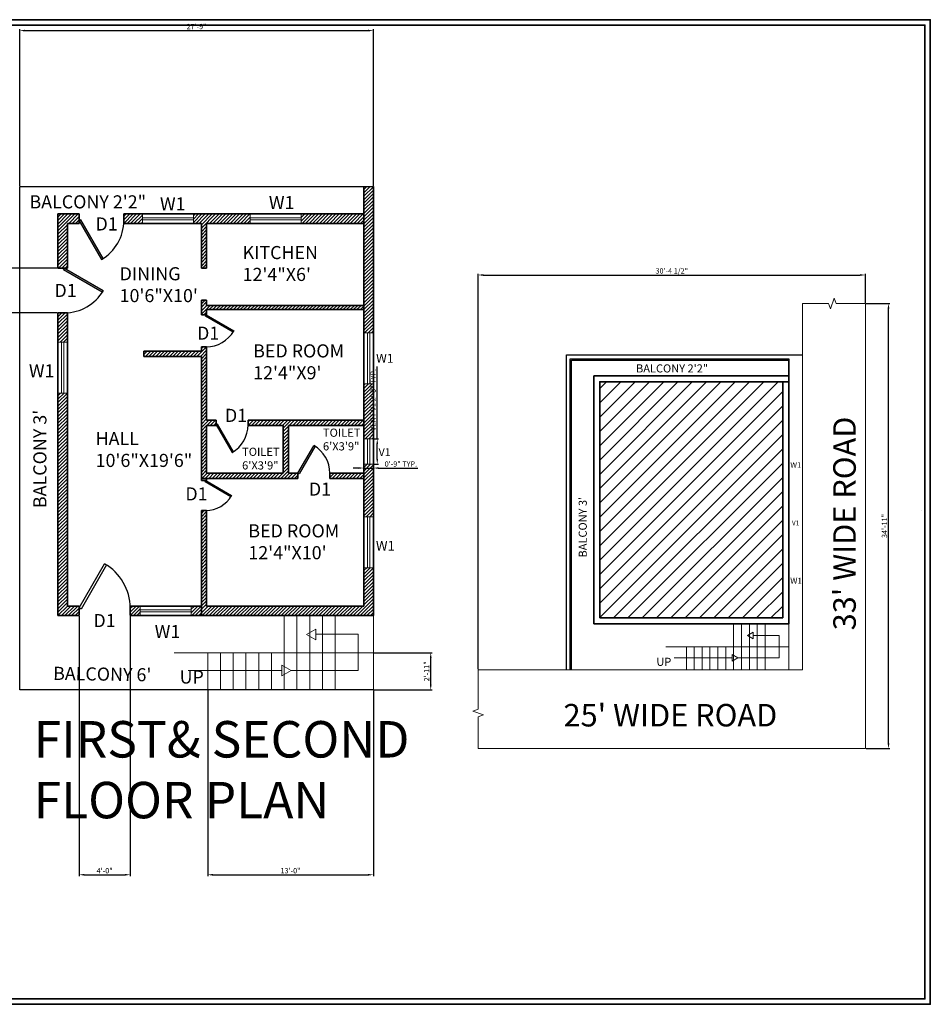
# Model space of a CAD drawing. Units: inches. Extents: x 2257 to 3849, y 1105 to 2032.
# Tile 2 of 2: x 2992 to 3849, y 1105 to 2032. Entities that reach past the tile are written whole.
import ezdxf

# ---------------------------------------------------------------- set-up
doc = ezdxf.new("R2010")
doc.units = ezdxf.units.IN
for name, color, linetype, lineweight in [('A-ANNO-DIMS', 7, 'Continuous', 18), ('A-ANNO-SYMB', 7, 'Continuous', 18), ('A-ANNO-TEXT', 130, 'Continuous', 18), ('A-ANNO-TTLB', 7, 'Continuous', 35), ('A-AREA-IDEN', 130, 'Continuous', 18), ('A-FLOR-OTLN', 7, 'Continuous', 25), ('C-PROP', 7, 'Continuous', 25), ('C-ROAD', 7, 'Continuous', 18), ('Doors', 100, 'Continuous', 25), ('steps', 220, 'Continuous', 18), ('walls', 10, 'Continuous', 35), ('windows', 160, 'Continuous', 18)]:
    doc.layers.add(name, color=color, linetype=linetype, lineweight=lineweight)
doc.layers.add('A-ROOF-PATT', color=51, linetype='Continuous', lineweight=13, true_color=0xf8f6b0)
doc.layers.add('A-WALL-PATT', color=241, linetype='Continuous', lineweight=13, true_color=0xf7abae)
doc.styles.get("Standard").update_dxf_attribs({"font": 'arial.ttf'})
doc.dimstyles.new('ISO-25', dxfattribs={"dimtxt": 5, "dimasz": 5, "dimexe": 1.25, "dimexo": 0.625, "dimtad": 1, "dimlunit": 3, "dimtxsty": 'Standard', "dimcen": 2.5, "dimadec": 0, "dimazin": 0, "dimtfac": 1, "dimtmove": 0, "dimatfit": 3, "dimfxl": 1, "dimarcsym": 0})
pattern_1 = [(45, (-85.9454, 0), (-1.6164461, 1.6164461), [])]

# ---------------------------------------------------------------- blocks, each defined once
blk = doc.blocks.new('*U4')
for p, q in [((0, 0), (0, -6)), ((40, 0), (40, -6))]:
    blk.add_line(p, q)
blk.add_lwpolyline([(0, 0), (20, 34.64), (21.52, 33.77), (1.52, -0.88)], close=True)
blk.add_arc((0, 0), 40, 0, 60)
blk = doc.blocks.new('*U5')
for p, q in [((-40, 0), (-40, 6)), ((0, 0), (0, 6))]:
    blk.add_line(p, q)
blk.add_lwpolyline([(0, 0), (-20, -34.64), (-21.52, -33.77), (-1.52, 0.87)], close=True)
blk.add_arc((0, 0), 40, 180, 240)
blk = doc.blocks.new('*U6')
for p, q in [((0, 0), (0, -6)), ((-40, 0), (-40, -6))]:
    blk.add_line(p, q)
blk.add_lwpolyline([(0, 0), (-20, 34.64), (-21.52, 33.77), (-1.52, -0.88)], close=True)
blk.add_arc((0, 0), 40, 120, 180)
blk = doc.blocks.new('*U7')
for p, q in [((-40, 0), (-40, 6)), ((0, 0), (0, 6))]:
    blk.add_line(p, q)
blk.add_lwpolyline([(0, 0), (-20, -34.6), (-21.5, -33.8), (-1.5, 0.9)], close=True)
blk.add_arc((0, 0), 40, 180, 240)
blk = doc.blocks.new('WIN-W1-48IN')
for p, q in [((0, 5.5), (48, 5.5)), ((0, 3.5), (48, 3.5))]:
    blk.add_line(p, q)
blk.add_lwpolyline([(0, 9), (48, 9), (48, 0), (0, 0)], close=True)
blk = doc.blocks.new('VENT-V1-24IN')
for p, q in [((3.5, 0), (3.5, 24)), ((5.5, 0), (5.5, 24))]:
    blk.add_line(p, q)
blk.add_lwpolyline([(0, 0), (0, 24), (9, 24), (9, 0)], close=True)
blk = doc.blocks.new('STAIR-DIRECTION-RETURN')
for points in [[(96.97, 5.1), (160.01, 5.1), (160.01, 39.11), (120.14, 39.11)], [(0, 5.1), (88.35, 5.1)]]:
    blk.add_lwpolyline(points)
for points in [[(120.14, 34.02), (120.14, 44.09), (111.42, 39.05)], [(88.35, 10.07), (88.35, 0), (97.07, 5.03)]]:
    blk.add_lwpolyline(points, close=True)
blk = doc.blocks.new('*D20')
at = {"layer": 'A-ANNO-DIMS', "color": 0, "lineweight": -2, "transparency": 16777216}
for p, q in [((3328.33, 1637.83), (3328.33, 1705.87)), ((3325.36, 1637.83), (3329.58, 1637.83)), ((3328.33, 1618.83), (3328.33, 1632.83)), ((3325.36, 1613.83), (3329.58, 1613.83))]:
    blk.add_line(p, q, dxfattribs=at)
at = {"layer": 'A-ANNO-DIMS', "color": 0, "transparency": 16777216}
for points in [[(3327.5, 1632.83), (3329.16, 1632.83), (3328.33, 1637.83)], [(3327.5, 1618.83), (3329.16, 1618.83), (3328.33, 1613.83)]]:
    blk.add_solid(points, dxfattribs=at)
at = {"layer": 'DEFPOINTS', "color": 0, "transparency": 16777216}
for p in [(3324.73, 1637.83), (3328.33, 1637.83), (3324.73, 1613.83)]:
    blk.add_point(p, dxfattribs=at)
at = {"layer": 'A-ANNO-DIMS', "color": 0, "transparency": 16777216, "insert": (3325.15, 1674.35), "char_height": 5, "attachment_point": 5, "rotation": 90}
blk.add_mtext('VENT V1 2\'-0" TYP.', dxfattribs=at)
blk = doc.blocks.new('*D21')
at = {"layer": 'A-ANNO-DIMS', "color": 0, "lineweight": -2, "transparency": 16777216}
for p, q in [((3315.73, 1613.2), (3315.73, 1608.98)), ((3324.73, 1613.2), (3324.73, 1608.98)), ((3310.73, 1610.23), (3305.73, 1610.23)), ((3315.73, 1610.23), (3324.73, 1610.23)), ((3329.73, 1610.23), (3366.46, 1610.23))]:
    blk.add_line(p, q, dxfattribs=at)
at = {"layer": 'A-ANNO-DIMS', "color": 0, "transparency": 16777216}
for points in [[(3310.73, 1611.06), (3310.73, 1609.39), (3315.73, 1610.23)], [(3329.73, 1611.06), (3329.73, 1609.39), (3324.73, 1610.23)]]:
    blk.add_solid(points, dxfattribs=at)
at = {"layer": 'DEFPOINTS', "color": 0, "transparency": 16777216}
for p in [(3315.73, 1613.83), (3324.73, 1613.83), (3324.73, 1610.23)]:
    blk.add_point(p, dxfattribs=at)
at = {"layer": 'A-ANNO-DIMS', "color": 0, "transparency": 16777216, "insert": (3350.6, 1613.4), "char_height": 5, "attachment_point": 5}
blk.add_mtext('0\'-9" TYP.', dxfattribs=at)
blk = doc.blocks.new('*D22')
at = {"layer": 'A-ANNO-DIMS', "color": 0, "lineweight": -2, "transparency": 16777216}
for p, q in [((2991.73, 1875.97), (2991.73, 2023.22)), ((2996.73, 2021.97), (3319.73, 2021.97)), ((3324.73, 1875.97), (3324.73, 2023.22))]:
    blk.add_line(p, q, dxfattribs=at)
at = {"layer": 'A-ANNO-DIMS', "color": 0, "transparency": 16777216}
for points in [[(2996.73, 2022.81), (2996.73, 2021.14), (2991.73, 2021.97)], [(3319.73, 2022.81), (3319.73, 2021.14), (3324.73, 2021.97)]]:
    blk.add_solid(points, dxfattribs=at)
at = {"layer": 'DEFPOINTS', "color": 0, "transparency": 16777216}
for p in [(3324.73, 2021.97), (2991.73, 1875.35), (3324.73, 1875.35)]:
    blk.add_point(p, dxfattribs=at)
at = {"layer": 'A-ANNO-DIMS', "color": 0, "transparency": 16777216, "insert": (3158.23, 2025.15), "char_height": 5, "attachment_point": 5}
blk.add_mtext('27\'-9"', dxfattribs=at)
blk = doc.blocks.new('*D24')
at = {"layer": 'A-ANNO-DIMS', "color": 0, "lineweight": -2, "transparency": 16777216}
for p, q in [((3047.73, 1470.72), (3047.73, 1226.15)), ((3095.73, 1470.72), (3095.73, 1226.15)), ((3052.73, 1227.4), (3090.73, 1227.4))]:
    blk.add_line(p, q, dxfattribs=at)
at = {"layer": 'A-ANNO-DIMS', "color": 0, "transparency": 16777216}
for points in [[(3052.73, 1228.23), (3052.73, 1226.56), (3047.73, 1227.4)], [(3090.73, 1228.23), (3090.73, 1226.56), (3095.73, 1227.4)]]:
    blk.add_solid(points, dxfattribs=at)
at = {"layer": 'DEFPOINTS', "color": 0, "transparency": 16777216}
for p in [(3047.73, 1471.35), (3095.73, 1471.35), (3095.73, 1227.4)]:
    blk.add_point(p, dxfattribs=at)
at = {"layer": 'A-ANNO-DIMS', "color": 0, "transparency": 16777216, "insert": (3071.73, 1230.57), "char_height": 5, "attachment_point": 5}
blk.add_mtext('4\'-0"', dxfattribs=at)
blk = doc.blocks.new('*D25')
at = {"layer": 'A-ANNO-DIMS', "color": 0, "lineweight": -2, "transparency": 16777216}
for p, q in [((3027.11, 1798.35), (2262.98, 1798.35)), ((2264.23, 1761.35), (2264.23, 1793.35)), ((3027.11, 1756.35), (2262.98, 1756.35))]:
    blk.add_line(p, q, dxfattribs=at)
at = {"layer": 'A-ANNO-DIMS', "color": 0, "transparency": 16777216}
for points in [[(2263.39, 1793.35), (2265.06, 1793.35), (2264.23, 1798.35)], [(2263.39, 1761.35), (2265.06, 1761.35), (2264.23, 1756.35)]]:
    blk.add_solid(points, dxfattribs=at)
at = {"layer": 'DEFPOINTS', "color": 0, "transparency": 16777216}
for p in [(2264.23, 1798.35), (3027.73, 1798.35), (3027.73, 1756.35)]:
    blk.add_point(p, dxfattribs=at)
at = {"layer": 'A-ANNO-DIMS', "color": 0, "transparency": 16777216, "insert": (2261.05, 1777.35), "char_height": 5, "attachment_point": 5, "rotation": 90}
blk.add_mtext('3\'-6"', dxfattribs=at)
blk = doc.blocks.new('*D28')
at = {"layer": 'A-ANNO-DIMS', "color": 0, "lineweight": -2, "transparency": 16777216}
for p, q in [((3168.73, 1400.72), (3168.73, 1226.15)), ((3324.73, 1400.72), (3324.73, 1226.15)), ((3173.73, 1227.4), (3319.73, 1227.4))]:
    blk.add_line(p, q, dxfattribs=at)
at = {"layer": 'A-ANNO-DIMS', "color": 0, "transparency": 16777216}
for points in [[(3173.73, 1228.23), (3173.73, 1226.56), (3168.73, 1227.4)], [(3319.73, 1228.23), (3319.73, 1226.56), (3324.73, 1227.4)]]:
    blk.add_solid(points, dxfattribs=at)
at = {"layer": 'DEFPOINTS', "color": 0, "transparency": 16777216}
for p in [(3168.73, 1401.35), (3324.73, 1401.35), (3324.73, 1227.4)]:
    blk.add_point(p, dxfattribs=at)
at = {"layer": 'A-ANNO-DIMS', "color": 0, "transparency": 16777216, "insert": (3246.73, 1230.58), "char_height": 5, "attachment_point": 5}
blk.add_mtext('13\'-0"', dxfattribs=at)
blk = doc.blocks.new('*D29')
at = {"layer": 'A-ANNO-DIMS', "color": 0, "lineweight": -2, "transparency": 16777216}
for p, q in [((3325.36, 1436.35), (3379.93, 1436.35)), ((3378.68, 1406.35), (3378.68, 1431.35)), ((3325.36, 1401.35), (3379.93, 1401.35))]:
    blk.add_line(p, q, dxfattribs=at)
at = {"layer": 'A-ANNO-DIMS', "color": 0, "transparency": 16777216}
for points in [[(3377.85, 1431.35), (3379.51, 1431.35), (3378.68, 1436.35)], [(3377.85, 1406.35), (3379.51, 1406.35), (3378.68, 1401.35)]]:
    blk.add_solid(points, dxfattribs=at)
at = {"layer": 'DEFPOINTS', "color": 0, "transparency": 16777216}
for p in [(3324.73, 1436.35), (3378.68, 1436.35), (3324.73, 1401.35)]:
    blk.add_point(p, dxfattribs=at)
at = {"layer": 'A-ANNO-DIMS', "color": 0, "transparency": 16777216, "insert": (3375.55, 1418.85), "char_height": 5, "attachment_point": 5, "rotation": 90}
blk.add_mtext('2\'-11"', dxfattribs=at)
blk = doc.blocks.new('*D30')
at = {"layer": 'A-ANNO-DIMS', "color": 0, "lineweight": -2, "transparency": 16777216}
for p, q in [((3423.28, 1420.92), (3423.28, 1793.17)), ((3428.28, 1791.92), (3782.92, 1791.92)), ((3787.92, 1765.76), (3787.92, 1793.17))]:
    blk.add_line(p, q, dxfattribs=at)
at = {"layer": 'A-ANNO-DIMS', "color": 0, "transparency": 16777216}
for points in [[(3428.28, 1792.76), (3428.28, 1791.09), (3423.28, 1791.92)], [(3782.92, 1792.76), (3782.92, 1791.09), (3787.92, 1791.92)]]:
    blk.add_solid(points, dxfattribs=at)
at = {"layer": 'DEFPOINTS', "color": 0, "transparency": 16777216}
for p in [(3787.92, 1791.92), (3787.92, 1765.13), (3423.28, 1420.3)]:
    blk.add_point(p, dxfattribs=at)
at = {"layer": 'A-ANNO-DIMS', "color": 0, "transparency": 16777216, "insert": (3605.6, 1795.14), "char_height": 5, "attachment_point": 5}
blk.add_mtext('30\'-4 1/2"', dxfattribs=at)
blk = doc.blocks.new('*D31')
at = {"layer": 'A-ANNO-DIMS', "color": 0, "lineweight": -2, "transparency": 16777216}
for p, q in [((3788.55, 1765.13), (3810.87, 1765.13)), ((3809.62, 1351.2), (3809.62, 1760.13)), ((3788.55, 1346.2), (3810.87, 1346.2))]:
    blk.add_line(p, q, dxfattribs=at)
at = {"layer": 'A-ANNO-DIMS', "color": 0, "transparency": 16777216}
for points in [[(3808.79, 1760.13), (3810.46, 1760.13), (3809.62, 1765.13)], [(3808.79, 1351.2), (3810.46, 1351.2), (3809.62, 1346.2)]]:
    blk.add_solid(points, dxfattribs=at)
at = {"layer": 'DEFPOINTS', "color": 0, "transparency": 16777216}
for p in [(3787.92, 1765.13), (3809.62, 1765.13), (3787.92, 1346.2)]:
    blk.add_point(p, dxfattribs=at)
at = {"layer": 'A-ANNO-DIMS', "color": 0, "transparency": 16777216, "insert": (3806.44, 1555.67), "char_height": 5, "attachment_point": 5, "rotation": 90}
blk.add_mtext('34\'-11"', dxfattribs=at)

msp = doc.modelspace()

# ---------------------------------------------------------------- hatches: boundary and pattern name
at = {"layer": 'A-ROOF-PATT'}
h = msp.add_hatch(dxfattribs=at)
h.set_pattern_fill('ANSI31', color=256, scale=3)
h.set_pattern_definition([(45, (-221.724, 0), (-6.735192, 6.735192), [])])
h.paths.add_polyline_path([(3710.119, 1469.082), (3710.119, 1691.383), (3537.836, 1691.383), (3537.836, 1665.448), (3537.836, 1469.082)])
at = {"layer": 'A-WALL-PATT'}
h = msp.add_hatch(dxfattribs=at)
h.set_pattern_fill('ANSI31', color=256, scale=0.72)
h.set_pattern_definition(pattern_1)
h.paths.add_polyline_path([(3036.731, 1840.347), (3047.731, 1840.347), (3047.731, 1849.347), (3027.731, 1849.347), (3027.731, 1798.347), (3036.731, 1798.347)])
h.paths.add_polyline_path([(3107.208, 1849.347), (3089.731, 1849.347), (3089.731, 1840.347), (3107.208, 1840.347)])
h.paths.add_polyline_path([(3208.789, 1849.347), (3155.208, 1849.347), (3155.208, 1840.347), (3162.731, 1840.347), (3162.731, 1798.347), (3167.731, 1798.347), (3167.731, 1840.347), (3208.789, 1840.347)])
h.paths.add_polyline_path([(3315.731, 1849.347), (3256.789, 1849.347), (3256.789, 1840.347), (3315.731, 1840.347)])
h.paths.add_polyline_path([(3324.731, 1875.347), (3315.731, 1875.347), (3315.731, 1737.469), (3324.731, 1737.469)])
h.paths.add_polyline_path([(3167.731, 1768.347), (3162.731, 1768.347), (3162.731, 1754.347), (3167.231, 1754.347), (3167.731, 1754.347), (3167.731, 1759.347), (3315.731, 1759.347), (3315.731, 1763.347), (3167.731, 1763.347)])
h.paths.add_polyline_path([(3167.731, 1724.347), (3162.731, 1724.347), (3162.731, 1720.347), (3108.731, 1720.347), (3108.731, 1715.347), (3162.731, 1715.347), (3162.731, 1600.347), (3167.731, 1600.347), (3253.731, 1600.347), (3253.731, 1605.347), (3244.731, 1605.347), (3244.731, 1650.347), (3315.731, 1650.347), (3315.731, 1655.347), (3206.731, 1655.347), (3206.731, 1650.347), (3239.731, 1650.347), (3239.731, 1605.347), (3167.731, 1605.347), (3167.731, 1650.347), (3176.731, 1650.347), (3176.731, 1655.347), (3167.731, 1655.347)])
h.paths.add_polyline_path([(3324.731, 1689.469), (3315.731, 1689.469), (3315.731, 1637.826), (3324.731, 1637.826)])
h.paths.add_polyline_path([(3315.731, 1605.347), (3283.731, 1605.347), (3283.731, 1600.347), (3315.731, 1600.347)], flags=17)
h.paths.add_polyline_path([(3324.731, 1613.826), (3315.731, 1613.826), (3315.731, 1564.439), (3324.731, 1564.439)])
h.paths.add_polyline_path([(3324.731, 1516.439), (3315.731, 1516.439), (3315.731, 1480.347), (3167.731, 1480.347), (3167.731, 1570.347), (3162.731, 1570.347), (3162.731, 1471.347), (3324.731, 1471.347)])
h.paths.add_polyline_path([(3162.731, 1480.347), (3153.231, 1480.347), (3153.231, 1471.347), (3162.731, 1471.347)])
h.paths.add_polyline_path([(3105.231, 1480.347), (3095.731, 1480.347), (3095.731, 1471.347), (3105.231, 1471.347)])
h = msp.add_hatch(dxfattribs=at)
h.set_pattern_fill('ANSI31', color=256, scale=0.72)
h.set_pattern_definition(pattern_1)
h.paths.add_polyline_path([(2551.998, 1559.347), (2542.498, 1559.347), (2542.498, 1550.347), (2551.998, 1550.347)])
h.paths.add_polyline_path([(2494.498, 1559.347), (2484.998, 1559.347), (2484.998, 1550.347), (2494.498, 1550.347)])
h.paths.add_polyline_path([(3036.731, 1680.812), (3027.731, 1680.812), (3027.731, 1471.347), (3047.694, 1471.347), (3047.694, 1478.53), (3047.731, 1480.347), (3036.731, 1480.347)])
h.paths.add_polyline_path([(3036.731, 1756.347), (3027.731, 1756.347), (3027.731, 1728.812), (3036.731, 1728.812)])
h = msp.add_hatch(dxfattribs=at)
h.set_pattern_fill('ANSI31', color=256, scale=0.72)
h.set_pattern_definition(pattern_1)
h.paths.add_polyline_path([(3036.731, 1756.347), (3027.731, 1756.347), (3027.731, 1728.812), (3036.731, 1728.812)])

# ---------------------------------------------------------------- linework, layer by layer
at = {"layer": 'A-ANNO-SYMB'}
for points in [[(3728.644, 1765.134), (3753.039, 1765.134), (3754.892, 1760.044), (3758.597, 1770.223), (3760.449, 1765.134), (3787.924, 1765.134)], [(3667.811, 1431.653), (3706.737, 1431.653), (3706.737, 1452.659), (3682.121, 1452.659)], [(3607.932, 1431.653), (3662.491, 1431.653)], [(3423.275, 1420.3), (3423.275, 1383.369), (3418.186, 1381.517), (3428.365, 1377.812), (3423.275, 1375.959), (3423.275, 1346.199)]]:
    msp.add_lwpolyline(points, dxfattribs=at)
for points in [[(3682.121, 1449.512), (3682.121, 1455.731), (3676.735, 1452.621)], [(3662.491, 1434.724), (3662.491, 1428.506), (3667.876, 1431.615)]]:
    msp.add_lwpolyline(points, close=True, dxfattribs=at)
at = {"layer": 'A-ANNO-TTLB'}
for points in [[(2257.449, 2032.239), (3848.988, 2032.239), (3848.988, 1105.467), (2257.449, 1105.467)], [(2262.449, 2027.239), (3843.988, 2027.239), (3843.988, 1110.467), (2262.449, 1110.467)]]:
    msp.add_lwpolyline(points, close=True, dxfattribs=at)
at = {"layer": 'A-FLOR-OTLN'}
for p, q in [((2991.731, 1875.347), (3324.731, 1875.347)), ((2991.731, 1401.347), (2991.731, 1875.347)), ((3510.048, 1420.3), (3510.048, 1712.996)), ((3510.048, 1712.996), (3715.677, 1712.996)), ((3324.731, 1401.347), (2991.731, 1401.347))]:
    msp.add_line(p, q, dxfattribs=at)
msp.add_lwpolyline([(3511.283, 1420.3), (3511.283, 1711.761), (3715.677, 1711.761)], dxfattribs=at)
at = {"layer": 'C-PROP'}
for p, q in [((3506.343, 1420.3), (3506.343, 1716.701)), ((3506.343, 1716.701), (3728.644, 1716.701))]:
    msp.add_line(p, q, dxfattribs=at)
at = {"layer": 'C-ROAD'}
for p, q in [((3728.644, 1765.134), (3728.644, 1420.3)), ((3787.924, 1765.134), (3787.924, 1346.199)), ((3728.644, 1420.3), (3423.275, 1420.3)), ((3787.924, 1346.199), (3423.275, 1346.199))]:
    msp.add_line(p, q, dxfattribs=at)
at = {"layer": 'steps'}
for p, q in [((3240.731, 1471.347), (3240.731, 1401.347)), ((3252.731, 1471.347), (3252.731, 1401.347)), ((3252.731, 1471.347), (3252.731, 1401.347)), ((3264.731, 1471.347), (3264.731, 1401.347)), ((3276.731, 1471.347), (3276.731, 1401.347)), ((3288.731, 1471.347), (3288.731, 1401.347)), ((3324.731, 1471.347), (3324.731, 1401.347)), ((3663.806, 1463.525), (3663.806, 1420.3)), ((3678.626, 1463.525), (3678.626, 1420.3)), ((3686.037, 1463.525), (3686.037, 1420.3)), ((3693.447, 1463.525), (3693.447, 1420.3)), ((3715.677, 1463.525), (3715.677, 1420.3)), ((3599.931, 1441.912), (3715.677, 1441.912)), ((3619.346, 1441.912), (3619.346, 1420.3)), ((3626.756, 1441.912), (3626.756, 1420.3)), ((3634.166, 1441.912), (3634.166, 1420.3)), ((3641.576, 1441.912), (3641.576, 1420.3)), ((3648.986, 1441.912), (3648.986, 1420.3)), ((3656.396, 1441.912), (3656.396, 1420.3)), ((3137.29, 1436.347), (3324.731, 1436.347)), ((3168.731, 1436.347), (3168.731, 1401.347)), ((3180.731, 1436.347), (3180.731, 1401.347)), ((3192.731, 1436.347), (3192.731, 1401.347)), ((3204.731, 1436.347), (3204.731, 1401.347)), ((3216.731, 1436.347), (3216.731, 1401.347)), ((3228.731, 1436.347), (3228.731, 1401.347))]:
    msp.add_line(p, q, dxfattribs=at)
msp.add_lwpolyline([(3671.216, 1463.525), (3671.216, 1420.3)], close=True, dxfattribs=at)
at = {"layer": 'walls'}
for p, q in [((3315.731, 1875.347), (3315.731, 1480.347)), ((3324.731, 1875.347), (3324.731, 1471.347)), ((3027.731, 1849.347), (3047.731, 1849.347)), ((3027.731, 1798.347), (3027.731, 1849.347)), ((3047.731, 1840.347), (3047.731, 1849.347)), ((3089.731, 1849.347), (3315.731, 1849.347)), ((3089.731, 1840.347), (3089.731, 1849.347)), ((3036.731, 1840.347), (3047.731, 1840.347)), ((3036.731, 1798.347), (3036.731, 1840.347)), ((3089.731, 1840.347), (3162.731, 1840.347)), ((3162.731, 1798.347), (3162.731, 1840.347)), ((3167.731, 1840.347), (3167.731, 1798.347)), ((3167.731, 1840.347), (3315.731, 1840.347)), ((3027.731, 1798.347), (3036.731, 1798.347)), ((3162.731, 1798.347), (3167.731, 1798.347)), ((3162.731, 1768.347), (3167.731, 1768.347)), ((3162.731, 1754.347), (3162.731, 1768.347)), ((3167.731, 1768.347), (3167.731, 1763.347)), ((3167.731, 1763.347), (3315.731, 1763.347)), ((3027.731, 1756.347), (3036.731, 1756.347)), ((3027.731, 1471.347), (3027.731, 1756.347)), ((3036.731, 1480.347), (3036.731, 1756.347)), ((3162.731, 1754.347), (3167.731, 1754.347)), ((3167.731, 1759.347), (3315.731, 1759.347)), ((3167.731, 1759.347), (3167.731, 1754.347)), ((3162.731, 1724.347), (3167.731, 1724.347)), ((3162.731, 1720.347), (3162.731, 1724.347)), ((3167.731, 1724.347), (3167.731, 1655.347)), ((3108.731, 1720.347), (3162.731, 1720.347)), ((3108.731, 1715.347), (3108.731, 1720.347)), ((3108.731, 1715.347), (3162.731, 1715.347)), ((3162.731, 1600.347), (3162.731, 1715.347)), ((3715.677, 1712.996), (3715.677, 1463.525)), ((3710.119, 1691.383), (3710.119, 1469.082)), ((3167.731, 1655.347), (3176.731, 1655.347)), ((3167.731, 1650.347), (3176.731, 1650.347)), ((3167.731, 1650.347), (3167.731, 1605.347)), ((3176.731, 1655.347), (3176.731, 1650.347)), ((3206.731, 1655.347), (3315.731, 1655.347)), ((3206.731, 1655.347), (3206.731, 1650.347)), ((3206.731, 1650.347), (3239.731, 1650.347)), ((3239.731, 1650.347), (3239.731, 1605.347)), ((3244.731, 1650.347), (3244.731, 1605.347)), ((3244.731, 1650.347), (3315.731, 1650.347)), ((3167.731, 1605.347), (3239.731, 1605.347)), ((3244.731, 1605.347), (3253.731, 1605.347)), ((3253.731, 1605.347), (3253.731, 1600.347)), ((3283.731, 1605.347), (3315.731, 1605.347)), ((3283.731, 1605.347), (3283.731, 1600.347)), ((3162.731, 1600.347), (3253.731, 1600.347)), ((3162.731, 1600.347), (3167.731, 1600.347)), ((3162.731, 1600.347), (3162.731, 1598.347)), ((3162.731, 1598.347), (3167.731, 1598.347)), ((3167.731, 1598.347), (3167.731, 1600.347)), ((3283.731, 1600.347), (3315.731, 1600.347)), ((3162.731, 1570.347), (3167.731, 1570.347)), ((3162.731, 1471.347), (3162.731, 1570.347)), ((3167.731, 1570.347), (3167.731, 1480.347)), ((3036.731, 1480.347), (3047.731, 1480.347)), ((3047.731, 1471.347), (3047.731, 1480.347)), ((3095.731, 1480.347), (3162.731, 1480.347)), ((3095.731, 1471.347), (3095.731, 1480.347)), ((3167.731, 1480.347), (3315.731, 1480.347)), ((3027.731, 1471.347), (3047.731, 1471.347)), ((3095.731, 1471.347), (3162.731, 1471.347)), ((3162.731, 1471.347), (3324.731, 1471.347)), ((3710.119, 1469.082), (3537.836, 1469.082)), ((3715.677, 1463.525), (3532.278, 1463.525))]:
    msp.add_line(p, q, dxfattribs=at)
for points in [[(3532.278, 1696.941), (3532.278, 1463.525)], [(3544.628, 1696.941), (3532.278, 1696.941), (3532.278, 1665.448)], [(3532.278, 1592.87), (3532.278, 1696.941)], [(3537.836, 1696.941), (3715.677, 1696.941)], [(3715.677, 1691.383), (3537.836, 1691.383)], [(3537.836, 1665.448), (3537.836, 1691.383), (3544.628, 1691.383)], [(3537.836, 1469.082), (3537.836, 1691.383)], [(3537.836, 1622.511), (3537.836, 1639.513)]]:
    msp.add_lwpolyline(points, dxfattribs=at)
at = {"layer": 'windows'}
for p, q in [((3031.231, 1680.812), (3031.231, 1728.812)), ((3033.231, 1680.812), (3033.231, 1728.812))]:
    msp.add_line(p, q, dxfattribs=at)
for points in [[(3027.731, 1680.812), (3027.731, 1728.812), (3036.731, 1728.812), (3036.731, 1680.812)], [(3840.593, 1570.605), (3840.593, 1570.605)]]:
    msp.add_lwpolyline(points, close=True, dxfattribs=at)

# ---------------------------------------------------------------- block references
at = {"layer": 'A-ANNO-SYMB'}
msp.add_blockref('STAIR-DIRECTION-RETURN', (3150.247, 1414.636), dxfattribs=at)
at = {"layer": 'Doors'}
for name, p, xscale, yscale, zscale, rotation in [('*U6', (3047.731, 1843.047), 1.049999999999999, 1.049999999999999, 1.049999999999999, 180), ('*U5', (3034.031, 1798.347), 1.049999999999999, 1.049999999999999, 1.049999999999999, 90), ('*U5', (3167.231, 1754.347), 0.75, 0.75, 0.75, 90), ('*U6', (3176.731, 1650.849), 0.7496246408594235, 0.7496246408594235, 0.7496246408594235, 180), ('*U7', (3253.731, 1605.347), 0.7496246408594235, 0.7496246408594235, 0.7496246408594235, 180), ('*U5', (3166.931, 1598.347), 0.6999999999999944, 0.6999999999999944, 0.6999999999999944, 90)]:
    msp.add_blockref(name, p, dxfattribs=dict(at, xscale=xscale, yscale=yscale, zscale=zscale, rotation=rotation))
at = {"layer": 'Doors', "xscale": 1.200942847219647, "yscale": 1.200942847219647, "zscale": 1.200942847219647}
msp.add_blockref('*U4', (3047.694, 1478.53), dxfattribs=at)
at = {"layer": 'windows'}
for name, p in [('WIN-W1-48IN', (3107.207, 1840.347)), ('WIN-W1-48IN', (3208.789, 1840.347)), ('VENT-V1-24IN', (3315.731, 1613.826)), ('WIN-W1-48IN', (3105.231, 1471.347))]:
    msp.add_blockref(name, p, dxfattribs=at)
for p, rotation in [((3324.731, 1689.469), 89.99999999999923), ((3324.731, 1516.439), 89.99999999999905)]:
    msp.add_blockref('WIN-W1-48IN', p, dxfattribs=dict(at, rotation=rotation))

# ---------------------------------------------------------------- texts
at = {"layer": 'A-ANNO-TEXT', "attachment_point": 1}
for s, width, gutter_width, insert, char_height in [('W1', 167.82029, 61.663, (3123.769, 1865.042), 12.3325), ('W1', 167.82029, 61.663, (3226.304, 1866.238), 12.3325), ('D1', 167.82029, 61.663, (3063.102, 1846.134), 12.3325), ('D1', 167.82029, 61.663, (3024.457, 1783.521), 12.3325), ('D1', 167.82029, 61.663, (3158.715, 1743.35), 12.3325), ('W1', 114.48409, 42.065, (3327.262, 1717.711), 8.413), ('W1', 167.82029, 61.663, (3000.401, 1707.912), 12.3325), ('D1', 167.82029, 61.663, (3184.947, 1665.964), 12.3325), ('V1', 100.10563, 36.782, (3329.599, 1628.888), 7.3564), ('W1', 70.69423, 25.975, (3717.24, 1615.655), 5.1951), ('D1', 167.82029, 61.663, (3263.962, 1596.568), 12.3325), ('D1', 167.82029, 61.663, (3147.704, 1592.042), 12.3325), ('V1', 61.8155, 22.713, (3718.682, 1560.807), 4.5426), ('W1', 124.29149, 45.669, (3327.091, 1541.615), 9.1337), ('W1', 76.75033, 28.201, (3717.134, 1506.916), 5.6401), ('D1', 167.82029, 61.663, (3061.139, 1472.812), 12.3325), ('W1', 167.82029, 61.663, (3118.81, 1462.459), 12.3325), ('UP', 103.62948, 38.077, (3591.126, 1431.653), 7.6154), ('UP', 167.82029, 61.663, (3142.281, 1419.732), 12.3325), ("25' WIDE ROAD", 288.40348, 105.969, (3503.733, 1388.191), 21.19372), ('FIRST& SECOND FLOOR PLAN', 467.04814, 171.608, (3004.915, 1372.061), 34.32167)]:
    msp.add_mtext_dynamic_manual_height_columns(s, width=width, gutter_width=gutter_width, heights=[0], dxfattribs=dict(at, insert=insert, char_height=char_height))
at = {"layer": 'A-ANNO-TEXT', "insert": (3757.627, 1457.47), "char_height": 21.19372, "attachment_point": 1, "rotation": 90}
msp.add_mtext_dynamic_manual_height_columns("33' WIDE ROAD", width=288.40348, gutter_width=105.969, heights=[0], dxfattribs=at)
at = {"layer": 'A-AREA-IDEN', "attachment_point": 1}
for s, width, gutter_width, insert, char_height in [('BALCONY 2\'2"', 254.30567, 61.663, (3000.93, 1866.935), 12.3325), ('KITCHEN \\P12\'4"X6\'', 167.82029, 61.663, (3201.588, 1819.217), 12.3325), ('DINING \\P10\'6"X10\'', 167.82029, 61.663, (3085.81, 1799.256), 12.3325), ('BED ROOM\\P12\'4"X9\'', 167.82029, 61.663, (3211.518, 1726.65), 12.3325), ('BALCONY 2\'2"', 157.03443, 38.077, (3571.956, 1707.802), 7.61535), ('HALL \\P10\'6"X19\'6"', 167.82029, 61.663, (3063.217, 1644.142), 12.3325), ('TOILET\\P6\'X3\'9"', 104.71521, 38.476, (3277.225, 1647.35), 7.6951), ('TOILET\\P6\'X3\'9"', 104.71521, 38.476, (3201.091, 1629.38), 7.6951), ('BED ROOM  \\P12\'4"X10\'', 167.82029, 61.663, (3206.987, 1557.279), 12.3325)]:
    msp.add_mtext_dynamic_manual_height_columns(s, width=width, gutter_width=gutter_width, heights=[0], dxfattribs=dict(at, insert=insert, char_height=char_height))
for s, width, gutter_width, insert, char_height, rotation in [("BALCONY 3'", 254.30567, 61.663, (3004.586, 1572.53), 12.3325, 90), ("BALCONY 3'", 157.03443, 38.077, (3517.986, 1526.006), 7.6154, 90), ("BALCONY 6'", 254.30567, 61.663, (3023.295, 1423.212), 12.3325, 359.068345)]:
    msp.add_mtext_dynamic_manual_height_columns(s, width=width, gutter_width=gutter_width, heights=[0], dxfattribs=dict(at, insert=insert, char_height=char_height, rotation=rotation))

# ---------------------------------------------------------------- dimensions: what is measured, and where the dimension line sits
at = {"layer": 'A-ANNO-DIMS'}
for base, p1, p2, picture, middle in [((3324.731, 2021.972), (2991.731, 1875.347), (3324.731, 1875.347), '*D22', (3158.231, 2025.15)), ((3787.924, 1791.923), (3423.275, 1420.3), (3787.924, 1765.134), '*D30', (3605.6, 1795.135)), ((3095.731, 1227.397), (3047.731, 1471.347), (3095.731, 1471.347), '*D24', (3071.731, 1230.574)), ((3324.731, 1227.397), (3168.731, 1401.347), (3324.731, 1401.347), '*D28', (3246.731, 1230.576))]:
    dim = msp.add_linear_dim(base=base, p1=p1, p2=p2, dimstyle='ISO-25', override={"dimdec": 1, "dimlfac": 1, "dimrnd": 0, "dimzin": 1, "dimdsep": 46, "dimlunit": 4, "dimfrac": 2}, dxfattribs=at)
    dim.commit()
    dim.dimension.update_dxf_attribs({"geometry": picture, "text_midpoint": middle})
for base, p1, p2, picture, middle in [((2264.228, 1798.347), (3027.731, 1756.347), (3027.731, 1798.347), '*D25', (2261.049, 1777.347)), ((3809.624, 1765.134), (3787.924, 1346.199), (3787.924, 1765.134), '*D31', (3806.445, 1555.666)), ((3378.681, 1436.347), (3324.731, 1401.347), (3324.731, 1436.347), '*D29', (3375.546, 1418.847))]:
    dim = msp.add_linear_dim(base=base, p1=p1, p2=p2, angle=90, dimstyle='ISO-25', override={"dimdec": 1, "dimlfac": 1, "dimrnd": 0, "dimzin": 1, "dimdsep": 46, "dimlunit": 4, "dimfrac": 2}, dxfattribs=at)
    dim.commit()
    dim.dimension.update_dxf_attribs({"geometry": picture, "text_midpoint": middle})
dim = msp.add_linear_dim(base=(3328.331, 1637.826), p1=(3324.731, 1613.826), p2=(3324.731, 1637.826), angle=90, text='VENT V1 <> TYP.', dimstyle='ISO-25', override={"dimdec": 1, "dimlfac": 1, "dimrnd": 0, "dimzin": 1, "dimdsep": 46, "dimlunit": 4, "dimfrac": 2}, dxfattribs=at)
dim.commit()
dim.dimension.update_dxf_attribs({"geometry": '*D20', "text_midpoint": (3325.153, 1674.346)})
dim = msp.add_linear_dim(base=(3324.731, 1610.226), p1=(3315.731, 1613.826), p2=(3324.731, 1613.826), text='<> TYP.', dimstyle='ISO-25', override={"dimdec": 1, "dimlfac": 1, "dimrnd": 0, "dimzin": 1, "dimdsep": 46, "dimlunit": 4, "dimfrac": 2}, dxfattribs=at)
dim.commit()
dim.dimension.update_dxf_attribs({"geometry": '*D21', "text_midpoint": (3350.595, 1613.404)})

doc.saveas('drawing.dxf')
